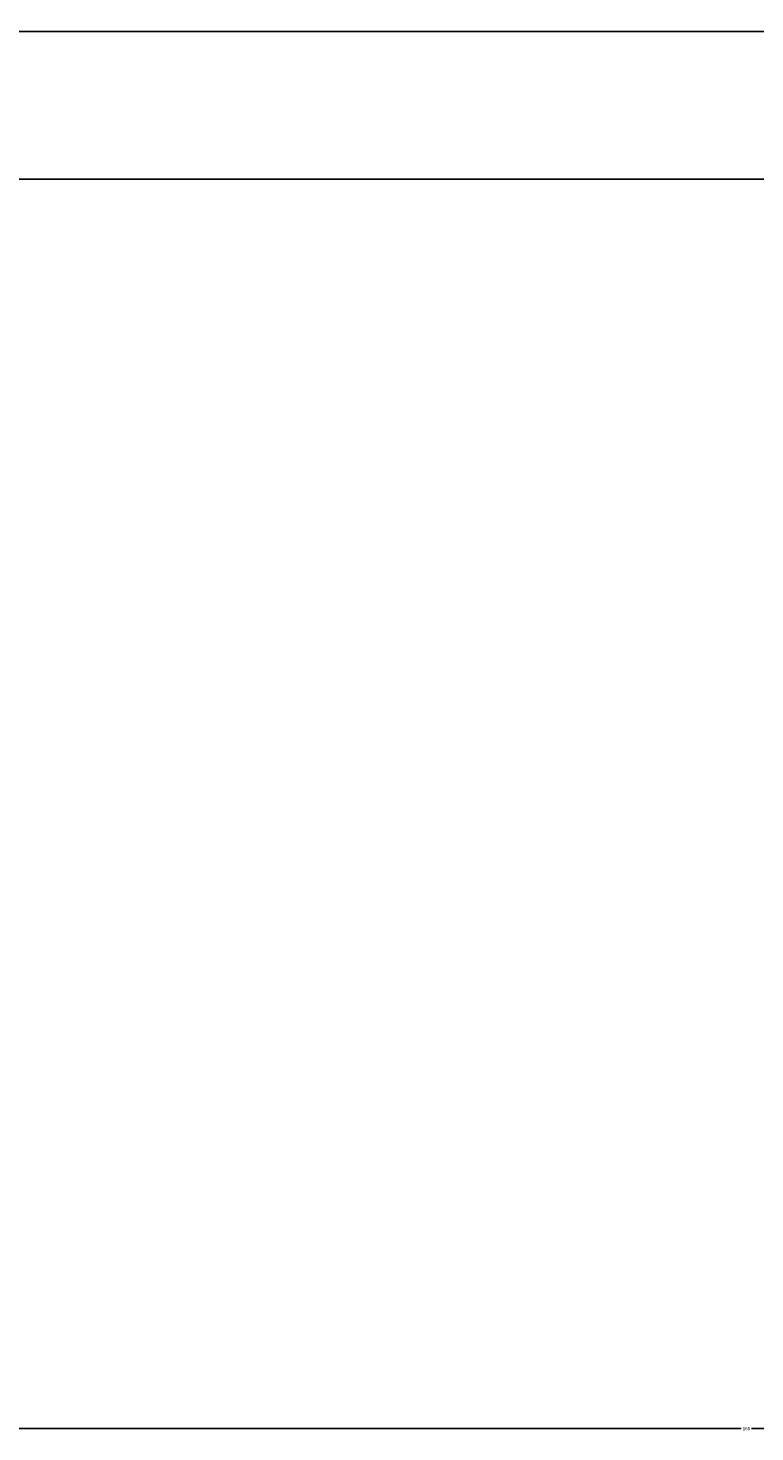
# Model space of a CAD drawing. Units: millimetres. Extents: x -48 to 129, y -118 to -41.
# Tile 5 of 6: x 1 to 40, y -118 to -41. Entities that reach past the tile are written whole.
import ezdxf

# ---------------------------------------------------------------- set-up
doc = ezdxf.new("R2010")
doc.units = ezdxf.units.MM
doc.layers.add('M-DIMS', color=2, linetype='Continuous', lineweight=18)
doc.styles.get("Standard").update_dxf_attribs({"font": 'arial.ttf'})
doc.dimstyles.get("Standard").update_dxf_attribs({"dimtxt": 0.18, "dimasz": 0.18, "dimexe": 0.18, "dimexo": 0.0625, "dimgap": 0.09, "dimtad": 0, "dimtih": 1, "dimtoh": 1, "dimdec": 4, "dimzin": 0, "dimdsep": 46, "dimtxsty": 'Standard', "dimcen": 0.09, "dimadec": 0, "dimazin": 0, "dimtfac": 1, "dimtdec": 4, "dimtofl": 0, "dimtmove": 0, "dimatfit": 3, "dimfxl": 1, "dimtolj": 1, "dimtzin": 0, "dimarcsym": 0})

# ---------------------------------------------------------------- blocks, each defined once
blk = doc.blocks.new('*D1')
at = {"layer": 'Defpoints', "color": 0, "transparency": 16777216}
for p in [(120, -79.442), (-40, -99.442), (120, -117.492)]:
    blk.add_point(p, dxfattribs=at)
at = {"layer": 'M-DIMS', "color": 0, "lineweight": -2, "transparency": 16777216}
for p, q in [((120, -79.505), (120, -117.672)), ((-40, -99.505), (-40, -117.672)), ((-39.82, -117.492), (39.72, -117.492)), ((119.82, -117.492), (40.28, -117.492))]:
    blk.add_line(p, q, dxfattribs=at)
at = {"layer": 'M-DIMS', "color": 0, "transparency": 16777216}
for points in [[(-39.82, -117.462), (-39.82, -117.522), (-40, -117.492)], [(119.82, -117.462), (119.82, -117.522), (120, -117.492)]]:
    blk.add_solid(points, dxfattribs=at)
at = {"layer": 'M-DIMS', "color": 0, "transparency": 16777216, "insert": (40, -117.492), "char_height": 0.18, "attachment_point": 5}
blk.add_mtext('\\A1;160', dxfattribs=at)
blk = doc.blocks.new('*D3')
at = {"layer": 'Defpoints', "color": 0, "transparency": 16777216}
for p in [(90, -41.392), (0, -59.442), (90, -79.442)]:
    blk.add_point(p, dxfattribs=at)
at = {"layer": 'M-DIMS', "color": 0, "lineweight": -2, "transparency": 16777216}
for p, q in [((0, -59.38), (0, -41.212)), ((90, -79.38), (90, -41.212)), ((0.18, -41.392), (44.781, -41.392)), ((89.82, -41.392), (45.219, -41.392))]:
    blk.add_line(p, q, dxfattribs=at)
at = {"layer": 'M-DIMS', "color": 0, "transparency": 16777216}
for points in [[(0.18, -41.362), (0.18, -41.422), (0, -41.392)], [(89.82, -41.362), (89.82, -41.422), (90, -41.392)]]:
    blk.add_solid(points, dxfattribs=at)
at = {"layer": 'M-DIMS', "color": 0, "transparency": 16777216, "insert": (45, -41.392), "char_height": 0.18, "attachment_point": 5}
blk.add_mtext('\\A1;90', dxfattribs=at)
blk = doc.blocks.new('*D8')
at = {"layer": 'Defpoints', "color": 0, "transparency": 16777216}
for p in [(-48.05, -49.442), (90, -49.442), (0, -59.442)]:
    blk.add_point(p, dxfattribs=at)
at = {"layer": 'M-DIMS', "color": 0, "lineweight": -2, "transparency": 16777216}
for p, q in [((89.938, -49.442), (-48.23, -49.442)), ((-48.05, -49.622), (-48.05, -54.26)), ((-48.05, -59.262), (-48.05, -54.624)), ((-0.062, -59.442), (-48.23, -59.442))]:
    blk.add_line(p, q, dxfattribs=at)
at = {"layer": 'M-DIMS', "color": 0, "transparency": 16777216}
for points in [[(-48.08, -49.622), (-48.02, -49.622), (-48.05, -49.442)], [(-48.08, -59.262), (-48.02, -59.262), (-48.05, -59.442)]]:
    blk.add_solid(points, dxfattribs=at)
at = {"layer": 'M-DIMS', "color": 0, "transparency": 16777216, "insert": (-48.05, -54.442), "char_height": 0.18, "attachment_point": 5}
blk.add_mtext('\\A1;10', dxfattribs=at)

msp = doc.modelspace()

# ---------------------------------------------------------------- dimensions: what is measured, and where the dimension line sits
at = {"layer": 'M-DIMS'}
for base, p1, p2, picture, middle in [((90, -41.392), (0, -59.442), (90, -79.442), '*D3', (45, -41.392)), ((120, -117.492), (-40, -99.442), (120, -79.442), '*D1', (40, -117.492))]:
    dim = msp.add_linear_dim(base=base, p1=p1, p2=p2, dimstyle='Standard', override={"dimdec": 0, "dimlfac": 1, "dimrnd": 0, "dimzin": 0, "dimdsep": 46, "dimlunit": 2}, dxfattribs=at)
    dim.commit()
    dim.dimension.update_dxf_attribs({"geometry": picture, "text_midpoint": middle})
dim = msp.add_linear_dim(base=(-48.05, -49.442), p1=(0, -59.442), p2=(90, -49.442), angle=90, dimstyle='Standard', override={"dimdec": 0, "dimlfac": 1, "dimrnd": 0, "dimzin": 0, "dimdsep": 46, "dimlunit": 2}, dxfattribs=at)
dim.commit()
dim.dimension.update_dxf_attribs({"geometry": '*D8', "text_midpoint": (-48.05, -54.442)})

doc.saveas('drawing.dxf')
